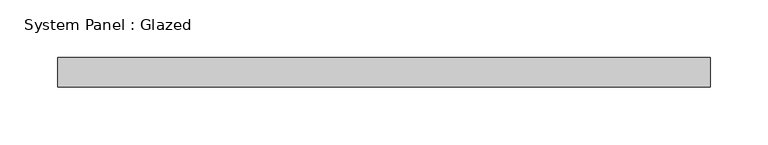
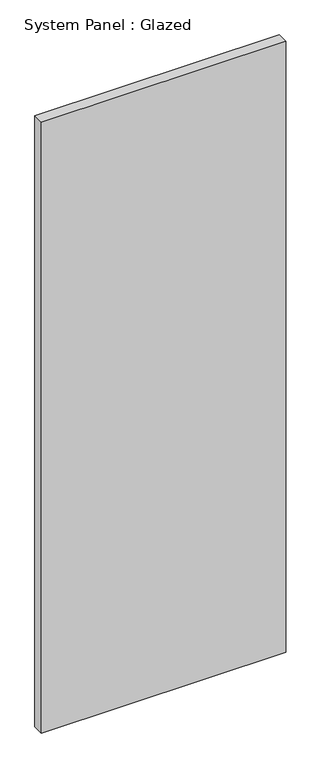
"""IFC4 building model written with IfcOpenShell, lengths in millimetres: plate geometry, System Panel : Glazed."""

from ifc_helpers import new_model, si_unit, origin, origin_with_axes, place, context, project, spatial, polyline, outline, extrude, source, transform, mapped, element, save


def system_panel_glazed_a8d9a87a(model_context):
    return source(origin(), model_context, "Body", "SweptSolid", [
        extrude(outline(polyline([(282.575, 19.05), (-282.575, 19.05), (-282.575, 44.45), (282.575, 44.45), (282.575, 19.05)])), origin_with_axes(), (0.0, 0.0, 1.0), 1492.7840707),
    ])


if __name__ == "__main__":
    model = new_model("IFC4")
    model_context = context("Model", 3, world=origin())
    ifc_project = project(units=[si_unit("LENGTHUNIT", "METRE", prefix="MILLI")], contexts=[model_context])
    site = spatial("IfcSite", under=ifc_project)
    building = spatial("IfcBuilding", under=site)
    placement = place(None, origin())
    system_panel_glazed_shape = system_panel_glazed_a8d9a87a(model_context)
    element("IfcPlate", 1, ObjectType="System Panel : Glazed", at=placement, inside=building, context=model_context, shape_type="MappedRepresentation", body=[
        mapped(system_panel_glazed_shape, transform((0.0, 0.0, 0.0), x_axis=(1.0, 0.0, 0.0), y_axis=(0.0, 1.0, 0.0), z_axis=(0.0, 0.0, 1.0))),
    ])
    save(model, "model.ifc")

# Revit data of these elements
# Type "System Panel : Glazed"
#   Construction Type Id = "GSP4R"
#   Analytic Construction = "1/8 in Pilkington single glazing"
#   Visual Light Transmittance = 0.9
#   Solar Heat Gain Coefficient = 0.86
#   Heat Transfer Coefficient (U) = 1.18115 BTU/(h·ft²·°F)
#   Define Thermal Properties by = 1
# Element 1 (IfcPlate, "System Panel : Glazed")
#   Materials on its faces: "Glass"
# Materials
#   "Glass": class "Glass", colour RGB 0 128 192, transparency 0.75, Description = "Soda Lime Glass", Cost = 0
